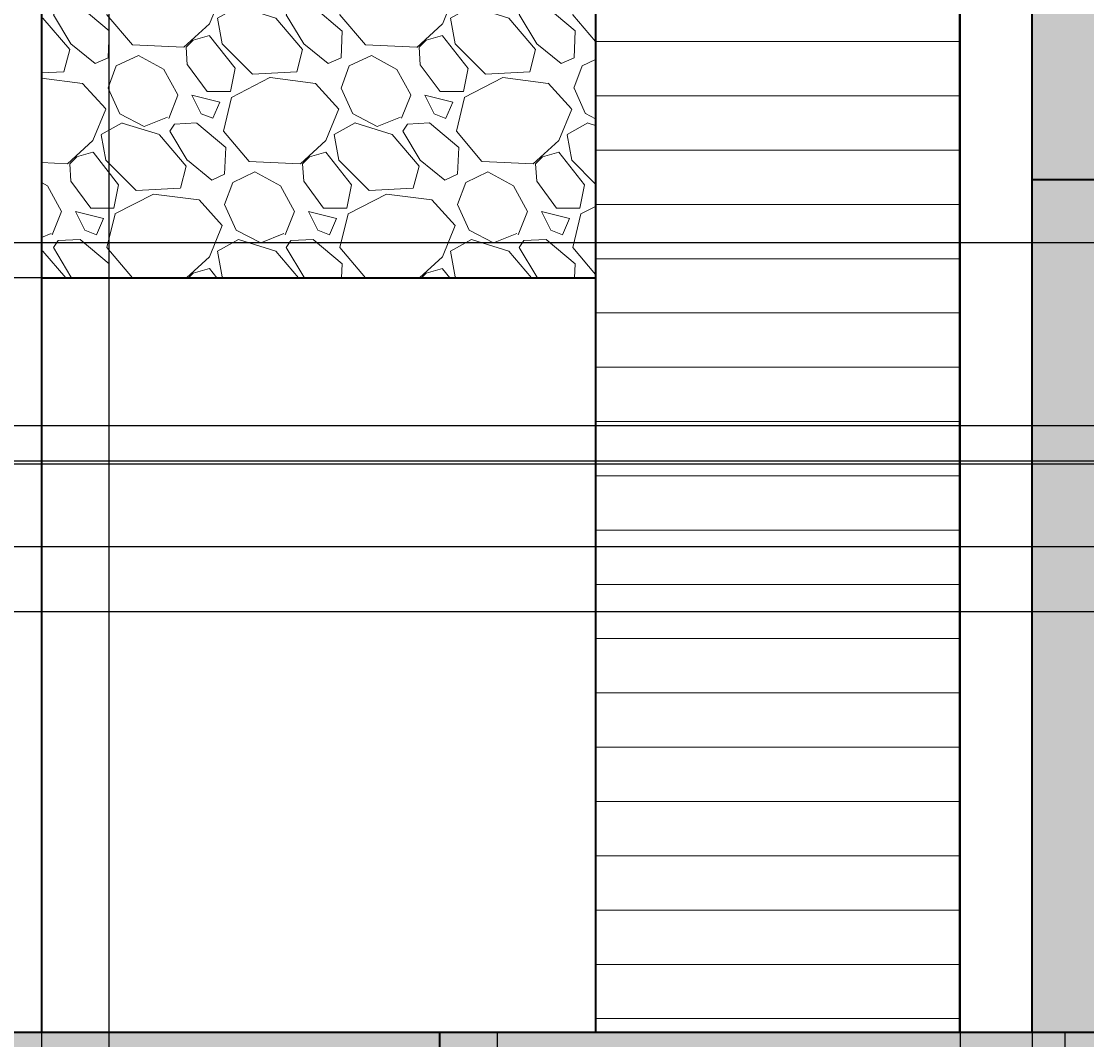
# Model space of a CAD drawing. Units: inches. Extents: x -5 to 714, y 84 to 644.
# Tile 4 of 20: x 124 to 266, y 200 to 336. Entities that reach past the tile are written whole.
import ezdxf

# ---------------------------------------------------------------- set-up
doc = ezdxf.new("R2010")
doc.units = ezdxf.units.IN
doc.header["$MEASUREMENT"] = 0
for name, color, linetype, lineweight in [('A-ANNO-DIMS', 2, 'Continuous', 18), ('A-ELEV', 7, 'Continuous', 35), ('A-ELEV-PATT', 8, 'Continuous', 13), ('A-GLAZ', 3, 'Continuous', 25)]:
    doc.layers.add(name, color=color, linetype=linetype, lineweight=lineweight)
doc.styles.get("Standard").update_dxf_attribs({"font": 'arial.ttf'})
doc.dimstyles.get("Standard").update_dxf_attribs({"dimtxt": 0.9375, "dimasz": 0.18, "dimexe": 0.18, "dimexo": 0.0625, "dimgap": 0.09, "dimtad": 0, "dimtih": 1, "dimtoh": 1, "dimdec": 4, "dimzin": 0, "dimdsep": 46, "dimlunit": 4, "dimtxsty": 'Standard', "dimcen": 0.09, "dimadec": 0, "dimazin": 0, "dimtfac": 1, "dimtdec": 4, "dimtofl": 0, "dimtmove": 0, "dimatfit": 3, "dimfxl": 1, "dimtolj": 1, "dimtzin": 0, "dimarcsym": 0})

# ---------------------------------------------------------------- blocks, each defined once
blk = doc.blocks.new('*D28')
at = {"layer": 'A-ANNO-DIMS', "color": 0, "lineweight": -2, "transparency": 16777216}
for p, q in [((126.73, 480.11), (126.73, 84.31)), ((135.73, 471.11), (135.73, 84.31)), ((126.91, 84.49), (130.83, 84.49)), ((135.55, 84.49), (131.63, 84.49))]:
    blk.add_line(p, q, dxfattribs=at)
at = {"layer": 'A-ANNO-DIMS', "color": 0, "transparency": 16777216}
for points in [[(126.91, 84.52), (126.91, 84.46), (126.73, 84.49)], [(135.55, 84.52), (135.55, 84.46), (135.73, 84.49)]]:
    blk.add_solid(points, dxfattribs=at)
at = {"layer": 'Defpoints', "color": 0, "transparency": 16777216}
for p in [(126.73, 480.17), (135.73, 471.17), (135.73, 84.49)]:
    blk.add_point(p, dxfattribs=at)
at = {"layer": 'A-ANNO-DIMS', "color": 0, "transparency": 16777216, "insert": (131.23, 84.49), "char_height": 0.938, "attachment_point": 5}
blk.add_mtext('\\A1;9', dxfattribs=at)
blk = doc.blocks.new('*D29')
at = {"layer": 'A-ANNO-DIMS', "color": 0, "lineweight": -2, "transparency": 16777216}
for p, q in [((135.73, 471.11), (135.73, 84.31)), ((429.51, 471.11), (429.51, 84.31)), ((135.91, 84.49), (280.94, 84.49)), ((429.33, 84.49), (284.3, 84.49))]:
    blk.add_line(p, q, dxfattribs=at)
at = {"layer": 'A-ANNO-DIMS', "color": 0, "transparency": 16777216}
for points in [[(135.91, 84.52), (135.91, 84.46), (135.73, 84.49)], [(429.33, 84.52), (429.33, 84.46), (429.51, 84.49)]]:
    blk.add_solid(points, dxfattribs=at)
at = {"layer": 'Defpoints', "color": 0, "transparency": 16777216}
for p in [(135.73, 471.17), (429.51, 471.17), (429.51, 84.49)]:
    blk.add_point(p, dxfattribs=at)
at = {"layer": 'A-ANNO-DIMS', "color": 0, "transparency": 16777216, "insert": (282.62, 84.49), "char_height": 0.938, "attachment_point": 5}
blk.add_mtext('\\A1;293.8', dxfattribs=at)
blk = doc.blocks.new('*D49')
at = {"layer": 'A-ANNO-DIMS', "color": 0, "lineweight": -2, "transparency": 16777216}
for p, q in [((126.73, 302), (126.73, 643.61)), ((126.91, 643.43), (162.98, 643.43)), ((200.56, 643.43), (164.49, 643.43)), ((200.74, 302), (200.74, 643.61))]:
    blk.add_line(p, q, dxfattribs=at)
at = {"layer": 'A-ANNO-DIMS', "color": 0, "transparency": 16777216}
for points in [[(126.91, 643.46), (126.91, 643.4), (126.73, 643.43)], [(200.56, 643.46), (200.56, 643.4), (200.74, 643.43)]]:
    blk.add_solid(points, dxfattribs=at)
at = {"layer": 'Defpoints', "color": 0, "transparency": 16777216}
for p in [(200.74, 643.43), (126.73, 301.94), (200.74, 301.94)]:
    blk.add_point(p, dxfattribs=at)
at = {"layer": 'A-ANNO-DIMS', "color": 0, "transparency": 16777216, "insert": (163.73, 643.43), "char_height": 0.938, "attachment_point": 5}
blk.add_mtext('\\A1;74', dxfattribs=at)
blk = doc.blocks.new('*D50')
at = {"layer": 'A-ANNO-DIMS', "color": 0, "lineweight": -2, "transparency": 16777216}
for p, q in [((200.67, 345.19), (-2.74, 345.19)), ((-2.56, 345.01), (-2.56, 324.13)), ((-2.56, 302.12), (-2.56, 323)), ((200.67, 301.94), (-2.74, 301.94))]:
    blk.add_line(p, q, dxfattribs=at)
at = {"layer": 'A-ANNO-DIMS', "color": 0, "transparency": 16777216}
for points in [[(-2.59, 345.01), (-2.53, 345.01), (-2.56, 345.19)], [(-2.59, 302.12), (-2.53, 302.12), (-2.56, 301.94)]]:
    blk.add_solid(points, dxfattribs=at)
at = {"layer": 'Defpoints', "color": 0, "transparency": 16777216}
for p in [(-2.56, 345.19), (200.74, 345.19), (200.74, 301.94)]:
    blk.add_point(p, dxfattribs=at)
at = {"layer": 'A-ANNO-DIMS', "color": 0, "transparency": 16777216, "insert": (-2.56, 323.57), "char_height": 0.938, "attachment_point": 5}
blk.add_mtext('\\A1;43.255', dxfattribs=at)
blk = doc.blocks.new('*D51')
at = {"layer": 'A-ANNO-DIMS', "color": 0, "lineweight": -2, "transparency": 16777216}
for p, q in [((200.74, 201.26), (200.74, 643.61)), ((200.92, 643.43), (223.39, 643.43)), ((249.24, 643.43), (226.77, 643.43)), ((249.42, 201.26), (249.42, 643.61))]:
    blk.add_line(p, q, dxfattribs=at)
at = {"layer": 'A-ANNO-DIMS', "color": 0, "transparency": 16777216}
for points in [[(200.92, 643.46), (200.92, 643.4), (200.74, 643.43)], [(249.24, 643.46), (249.24, 643.4), (249.42, 643.43)]]:
    blk.add_solid(points, dxfattribs=at)
at = {"layer": 'Defpoints', "color": 0, "transparency": 16777216}
for p in [(249.42, 643.43), (200.74, 201.19), (249.42, 201.19)]:
    blk.add_point(p, dxfattribs=at)
at = {"layer": 'A-ANNO-DIMS', "color": 0, "transparency": 16777216, "insert": (225.08, 643.43), "char_height": 0.938, "attachment_point": 5}
blk.add_mtext('\\A1;48.68', dxfattribs=at)
blk = doc.blocks.new('*D52')
at = {"layer": 'A-ANNO-DIMS', "color": 0, "lineweight": -2, "transparency": 16777216}
for p, q in [((249.42, 345.13), (249.42, 84.31)), ((259.07, 345.13), (259.07, 84.31)), ((249.6, 84.49), (252.57, 84.49)), ((258.89, 84.49), (255.92, 84.49))]:
    blk.add_line(p, q, dxfattribs=at)
at = {"layer": 'A-ANNO-DIMS', "color": 0, "transparency": 16777216}
for points in [[(249.6, 84.52), (249.6, 84.46), (249.42, 84.49)], [(258.89, 84.52), (258.89, 84.46), (259.07, 84.49)]]:
    blk.add_solid(points, dxfattribs=at)
at = {"layer": 'Defpoints', "color": 0, "transparency": 16777216}
for p in [(249.42, 345.19), (259.07, 345.19), (259.07, 84.49)]:
    blk.add_point(p, dxfattribs=at)
at = {"layer": 'A-ANNO-DIMS', "color": 0, "transparency": 16777216, "insert": (254.24, 84.49), "char_height": 0.938, "attachment_point": 5}
blk.add_mtext('\\A1;9.648', dxfattribs=at)
blk = doc.blocks.new('*D53')
at = {"layer": 'A-ANNO-DIMS', "color": 0, "lineweight": -2, "transparency": 16777216}
for p, q in [((259.07, 315.03), (259.07, 84.31)), ((269.24, 306.57), (269.24, 84.31)), ((259.25, 84.49), (262.16, 84.49)), ((269.06, 84.49), (266.15, 84.49))]:
    blk.add_line(p, q, dxfattribs=at)
at = {"layer": 'A-ANNO-DIMS', "color": 0, "transparency": 16777216}
for points in [[(259.25, 84.52), (259.25, 84.46), (259.07, 84.49)], [(269.06, 84.52), (269.06, 84.46), (269.24, 84.49)]]:
    blk.add_solid(points, dxfattribs=at)
at = {"layer": 'Defpoints', "color": 0, "transparency": 16777216}
for p in [(259.07, 315.1), (269.24, 306.63), (269.24, 84.49)]:
    blk.add_point(p, dxfattribs=at)
at = {"layer": 'A-ANNO-DIMS', "color": 0, "transparency": 16777216, "insert": (264.16, 84.49), "char_height": 0.938, "attachment_point": 5}
blk.add_mtext('\\A1;10.178', dxfattribs=at)
blk = doc.blocks.new('*D54')
at = {"layer": 'A-ANNO-DIMS', "color": 0, "lineweight": -2, "transparency": 16777216}
for p, q in [((259.07, 315.16), (259.07, 643.61)), ((259.25, 643.43), (424.21, 643.43)), ((593.25, 643.43), (428.28, 643.43)), ((593.43, 315.16), (593.43, 643.61))]:
    blk.add_line(p, q, dxfattribs=at)
at = {"layer": 'A-ANNO-DIMS', "color": 0, "transparency": 16777216}
for points in [[(259.25, 643.46), (259.25, 643.4), (259.07, 643.43)], [(593.25, 643.46), (593.25, 643.4), (593.43, 643.43)]]:
    blk.add_solid(points, dxfattribs=at)
at = {"layer": 'Defpoints', "color": 0, "transparency": 16777216}
for p in [(593.43, 643.43), (259.07, 315.1), (593.43, 315.1)]:
    blk.add_point(p, dxfattribs=at)
at = {"layer": 'A-ANNO-DIMS', "color": 0, "transparency": 16777216, "insert": (426.25, 643.43), "char_height": 0.938, "attachment_point": 5}
blk.add_mtext('\\A1;334.36', dxfattribs=at)
blk = doc.blocks.new('*D56')
at = {"layer": 'A-ANNO-DIMS', "color": 0, "lineweight": -2, "transparency": 16777216}
for p, q in [((578.03, 277.05), (-2.74, 277.05)), ((-2.56, 276.87), (-2.56, 239.69)), ((-2.56, 201.37), (-2.56, 238.55)), ((578.03, 201.19), (-2.74, 201.19))]:
    blk.add_line(p, q, dxfattribs=at)
at = {"layer": 'A-ANNO-DIMS', "color": 0, "transparency": 16777216}
for points in [[(-2.59, 276.87), (-2.53, 276.87), (-2.56, 277.05)], [(-2.59, 201.37), (-2.53, 201.37), (-2.56, 201.19)]]:
    blk.add_solid(points, dxfattribs=at)
at = {"layer": 'Defpoints', "color": 0, "transparency": 16777216}
for p in [(-2.56, 277.05), (578.09, 277.05), (578.09, 201.19)]:
    blk.add_point(p, dxfattribs=at)
at = {"layer": 'A-ANNO-DIMS', "color": 0, "transparency": 16777216, "insert": (-2.56, 239.12), "char_height": 0.938, "attachment_point": 5}
blk.add_mtext('\\A1;75.86', dxfattribs=at)
blk = doc.blocks.new('*D57')
at = {"layer": 'A-ANNO-DIMS', "color": 0, "lineweight": -2, "transparency": 16777216}
for p, q in [((578.03, 306.63), (-2.74, 306.63)), ((-2.56, 306.45), (-2.56, 292.41)), ((-2.56, 277.23), (-2.56, 291.27)), ((578.03, 277.05), (-2.74, 277.05))]:
    blk.add_line(p, q, dxfattribs=at)
at = {"layer": 'A-ANNO-DIMS', "color": 0, "transparency": 16777216}
for points in [[(-2.59, 306.45), (-2.53, 306.45), (-2.56, 306.63)], [(-2.59, 277.23), (-2.53, 277.23), (-2.56, 277.05)]]:
    blk.add_solid(points, dxfattribs=at)
at = {"layer": 'Defpoints', "color": 0, "transparency": 16777216}
for p in [(578.09, 306.63), (-2.56, 277.05), (578.09, 277.05)]:
    blk.add_point(p, dxfattribs=at)
at = {"layer": 'A-ANNO-DIMS', "color": 0, "transparency": 16777216, "insert": (-2.56, 291.84), "char_height": 0.938, "attachment_point": 5}
blk.add_mtext('\\A1;29.58', dxfattribs=at)
blk = doc.blocks.new('*D59')
at = {"layer": 'A-ANNO-DIMS', "color": 0, "lineweight": -2, "transparency": 16777216}
for p, q in [((593.37, 282.2), (-2.74, 282.2)), ((-2.56, 282.02), (-2.56, 280.41)), ((-2.56, 277.66), (-2.56, 279.27)), ((593.37, 277.48), (-2.74, 277.48))]:
    blk.add_line(p, q, dxfattribs=at)
at = {"layer": 'A-ANNO-DIMS', "color": 0, "transparency": 16777216}
for points in [[(-2.59, 282.02), (-2.53, 282.02), (-2.56, 282.2)], [(-2.59, 277.66), (-2.53, 277.66), (-2.56, 277.48)]]:
    blk.add_solid(points, dxfattribs=at)
at = {"layer": 'Defpoints', "color": 0, "transparency": 16777216}
for p in [(-2.56, 282.2), (593.43, 282.2), (593.43, 277.48)]:
    blk.add_point(p, dxfattribs=at)
at = {"layer": 'A-ANNO-DIMS', "color": 0, "transparency": 16777216, "insert": (-2.56, 279.84), "char_height": 0.938, "attachment_point": 5}
blk.add_mtext('\\A1;4.719', dxfattribs=at)
blk = doc.blocks.new('*D65')
at = {"layer": 'A-ANNO-DIMS', "color": 0, "lineweight": -2, "transparency": 16777216}
for p, q in [((325.77, 266), (-2.74, 266)), ((-2.56, 265.82), (-2.56, 219.13)), ((-2.56, 171.3), (-2.56, 217.99)), ((325.77, 171.12), (-2.74, 171.12))]:
    blk.add_line(p, q, dxfattribs=at)
at = {"layer": 'A-ANNO-DIMS', "color": 0, "transparency": 16777216}
for points in [[(-2.59, 265.82), (-2.53, 265.82), (-2.56, 266)], [(-2.59, 171.3), (-2.53, 171.3), (-2.56, 171.12)]]:
    blk.add_solid(points, dxfattribs=at)
at = {"layer": 'Defpoints', "color": 0, "transparency": 16777216}
for p in [(-2.56, 266), (325.83, 266), (325.83, 171.12)]:
    blk.add_point(p, dxfattribs=at)
at = {"layer": 'A-ANNO-DIMS', "color": 0, "transparency": 16777216, "insert": (-2.56, 218.56), "char_height": 0.938, "attachment_point": 5}
blk.add_mtext('\\A1;94.88', dxfattribs=at)
blk = doc.blocks.new('*D71')
at = {"layer": 'A-ANNO-DIMS', "color": 0, "lineweight": -2, "transparency": 16777216}
for p, q in [((537.12, 257.34), (-2.74, 257.34)), ((-2.56, 257.16), (-2.56, 229.83)), ((-2.56, 201.37), (-2.56, 228.7)), ((537.12, 201.19), (-2.74, 201.19))]:
    blk.add_line(p, q, dxfattribs=at)
at = {"layer": 'A-ANNO-DIMS', "color": 0, "transparency": 16777216}
for points in [[(-2.59, 257.16), (-2.53, 257.16), (-2.56, 257.34)], [(-2.59, 201.37), (-2.53, 201.37), (-2.56, 201.19)]]:
    blk.add_solid(points, dxfattribs=at)
at = {"layer": 'Defpoints', "color": 0, "transparency": 16777216}
for p in [(-2.56, 257.34), (537.18, 257.34), (537.18, 201.19)]:
    blk.add_point(p, dxfattribs=at)
at = {"layer": 'A-ANNO-DIMS', "color": 0, "transparency": 16777216, "insert": (-2.56, 229.27), "char_height": 0.938, "attachment_point": 5}
blk.add_mtext('\\A1;56.15', dxfattribs=at)
blk = doc.blocks.new('*D72')
at = {"layer": 'A-ANNO-DIMS', "color": 0, "lineweight": -2, "transparency": 16777216}
for p, q in [((493.71, 266), (-2.74, 266)), ((-2.56, 265.82), (-2.56, 234.17)), ((-2.56, 201.37), (-2.56, 233.03)), ((493.71, 201.19), (-2.74, 201.19))]:
    blk.add_line(p, q, dxfattribs=at)
at = {"layer": 'A-ANNO-DIMS', "color": 0, "transparency": 16777216}
for points in [[(-2.59, 265.82), (-2.53, 265.82), (-2.56, 266)], [(-2.59, 201.37), (-2.53, 201.37), (-2.56, 201.19)]]:
    blk.add_solid(points, dxfattribs=at)
at = {"layer": 'Defpoints', "color": 0, "transparency": 16777216}
for p in [(-2.56, 266), (493.78, 266), (493.78, 201.19)]:
    blk.add_point(p, dxfattribs=at)
at = {"layer": 'A-ANNO-DIMS', "color": 0, "transparency": 16777216, "insert": (-2.56, 233.6), "char_height": 0.938, "attachment_point": 5}
blk.add_mtext('\\A1;64.81', dxfattribs=at)
blk = doc.blocks.new('*D82')
at = {"layer": 'A-ANNO-DIMS', "color": 0, "lineweight": -2, "transparency": 16777216}
for p, q in [((263.37, 201.19), (-2.74, 201.19)), ((-2.56, 201.01), (-2.56, 177.22)), ((-2.56, 152.3), (-2.56, 176.09)), ((263.37, 152.12), (-2.74, 152.12))]:
    blk.add_line(p, q, dxfattribs=at)
at = {"layer": 'A-ANNO-DIMS', "color": 0, "transparency": 16777216}
for points in [[(-2.59, 201.01), (-2.53, 201.01), (-2.56, 201.19)], [(-2.59, 152.3), (-2.53, 152.3), (-2.56, 152.12)]]:
    blk.add_solid(points, dxfattribs=at)
at = {"layer": 'Defpoints', "color": 0, "transparency": 16777216}
for p in [(-2.56, 201.19), (263.43, 201.19), (263.43, 152.12)]:
    blk.add_point(p, dxfattribs=at)
at = {"layer": 'A-ANNO-DIMS', "color": 0, "transparency": 16777216, "insert": (-2.56, 176.66), "char_height": 0.938, "attachment_point": 5}
blk.add_mtext('\\A1;49.08', dxfattribs=at)

msp = doc.modelspace()

# ---------------------------------------------------------------- hatches: boundary and pattern name
at = {"layer": 'A-ELEV-PATT', "transparency": 33554687}
h = msp.add_hatch(color=256, dxfattribs=at)
h.dxf.hatch_style = 1
h.paths.add_polyline_path([(188.3677, 525.1928), (67.9893, 525.1928), (67.9893, 489.1928), (67.9893, 345.1928), (126.7303, 345.1928), (126.7303, 480.1709), (229.3575, 480.1709), (229.3575, 525.1928), (212.6043, 525.1928), (212.6043, 482.7164), (211.0019, 482.7164), (211.0019, 525.1928), (207.6919, 525.1928), (199.9852, 525.1928), (199.9852, 482.7164), (198.3828, 482.7164), (198.3828, 525.1928), (189.9701, 525.1928), (189.9701, 482.7164), (188.3677, 482.7164)])
h.paths.add_polyline_path([(121.3589, 336.2066), (75.5048, 336.2066), (75.5048, 319.345), (121.3589, 319.345)])
h.paths.add_polyline_path([(121.3589, 319.345), (75.5048, 319.345), (75.5048, 302.3045), (121.3589, 302.3045)])
h.paths.add_polyline_path([(121.3589, 302.3045), (75.5048, 302.3045), (75.5048, 282.8561), (121.3589, 282.8561)])
h.paths.add_polyline_path([(121.3589, 282.8561), (75.5048, 282.8561), (75.5048, 261.5556), (121.3589, 261.5556)])
h.paths.add_polyline_path([(121.3589, 261.5556), (75.5048, 261.5556), (75.5048, 243.7009), (121.3589, 243.7009)])
h.paths.add_polyline_path([(121.3589, 243.7009), (75.5048, 243.7009), (75.5048, 223.5117), (121.3589, 223.5117)])
h.paths.add_polyline_path([(121.3589, 223.5117), (75.5048, 223.5117), (75.5048, 212.5836), (121.3589, 212.5836)])
h.paths.add_polyline_path([(121.3589, 212.5836), (75.5048, 212.5836), (75.5048, 201.1928), (121.3589, 201.1928)])
h.paths.add_polyline_path([(179.9335, 201.1928), (30.1395, 201.1928), (30.1395, 198.7054), (179.9335, 198.7054)])
h.paths.add_polyline_path([(187.6349, 201.1928), (179.9335, 201.1928), (179.9335, 198.7054), (179.9335, 141.1928), (269.2446, 141.1928), (269.2446, 201.1928), (263.4349, 201.1928), (263.4349, 152.1176), (187.6349, 152.1176)])
h.paths.add_polyline_path([(269.2446, 277.0513), (269.2446, 287.501), (269.2446, 306.6286), (578.0915, 306.6286), (578.0915, 201.1928), (593.428, 201.1928), (593.428, 315.0968), (584.4202, 315.0968), (259.0665, 315.0968), (259.0665, 201.1928), (263.4349, 201.1928), (269.2446, 201.1928)])
h = msp.add_hatch(dxfattribs=at)
h.set_pattern_fill('ANSI31', color=256, scale=58, angle=135)
h.paths.add_polyline_path([(249.4181, 345.1928), (237.2654, 345.1928), (200.7361, 345.1928), (200.7361, 201.1928), (249.4181, 201.1928)])
h.paths.add_polyline_path([(261.4349, 199.1928), (189.6349, 199.1928), (189.6349, 154.1176), (261.4349, 154.1176)])
h.paths.add_polyline_path([(415.8092, 525.1928), (366.2809, 525.1928), (366.2809, 480.1709), (415.8092, 480.1709)])
h = msp.add_hatch(dxfattribs=at)
h.set_pattern_fill('GRAVEL', color=256, scale=22, angle=135)
h.paths.add_polyline_path([(200.7361, 345.1928), (126.7303, 345.1928), (126.7303, 301.9374), (200.7361, 301.9374)])
h = msp.add_hatch(color=256, dxfattribs=at)
h.dxf.hatch_style = 1
h.paths.add_polyline_path([(584.2229, 343.1928), (259.0665, 343.1928), (259.0665, 315.0968), (584.2229, 315.0968)])
h.paths.add_polyline_path([(352.9482, 258.2864), (332.0052, 258.2864), (332.0052, 201.1928), (352.9482, 201.1928)])
h.paths.add_polyline_path([(378.5957, 258.2864), (357.6527, 258.2864), (357.6527, 201.1928), (378.5957, 201.1928)])
h.paths.add_polyline_path([(403.4391, 258.2864), (382.4961, 258.2864), (382.4961, 201.1928), (403.4391, 201.1928)])
h.paths.add_polyline_path([(339.2672, 197.3754), (332.0052, 197.3754), (332.0052, 191.3028), (339.2672, 191.3028)])
h.paths.add_polyline_path([(352.9482, 197.3754), (343.9704, 197.3754), (343.9704, 191.3028), (352.9482, 191.3028)])
h.paths.add_polyline_path([(352.9482, 189.3028), (343.9704, 189.3028), (343.9704, 184.8307), (352.9482, 184.8307)])
h.paths.add_polyline_path([(339.2672, 189.3028), (332.0052, 189.3028), (332.0052, 184.8307), (339.2672, 184.8307)])
h.paths.add_polyline_path([(339.2672, 182.8307), (332.0052, 182.8307), (332.0052, 177.6504), (339.2672, 177.6504)])
h.paths.add_polyline_path([(352.9482, 182.8307), (343.9704, 182.8307), (343.9704, 177.6504), (352.9482, 177.6504)])
h.paths.add_polyline_path([(352.9482, 175.6504), (343.9704, 175.6504), (343.9704, 173.6169), (352.9482, 173.6169)])
h.paths.add_polyline_path([(339.2672, 175.6504), (332.0052, 175.6504), (332.0052, 173.6169), (339.2672, 173.6169)])
h.paths.add_polyline_path([(376.2796, 175.6504), (357.6527, 175.6504), (357.6527, 173.6169), (376.2796, 173.6169)])
h.paths.add_polyline_path([(376.2796, 182.8307), (357.6527, 182.8307), (357.6527, 177.6504), (376.2796, 177.6504)])
h.paths.add_polyline_path([(376.2796, 189.3028), (357.6527, 189.3028), (357.6527, 184.8307), (376.2796, 184.8307)])
h.paths.add_polyline_path([(376.2796, 197.3754), (357.6527, 197.3754), (357.6527, 191.3028), (376.2796, 191.3028)])
h.paths.add_polyline_path([(403.4391, 197.3754), (382.4961, 197.3754), (382.4961, 191.3028), (403.4391, 191.3028)])
h.paths.add_polyline_path([(403.4391, 189.3028), (382.4961, 189.3028), (382.4961, 184.8307), (403.4391, 184.8307)])
h.paths.add_polyline_path([(403.4391, 182.8307), (382.4961, 182.8307), (382.4961, 177.6504), (403.4391, 177.6504)])
h.paths.add_polyline_path([(403.4391, 175.6504), (382.4961, 175.6504), (382.4961, 173.6169), (403.4391, 173.6169)])
h = msp.add_hatch(color=256, dxfattribs=at)
h.dxf.hatch_style = 1
h.paths.add_polyline_path([(263.4349, 201.1928), (187.6349, 201.1928), (187.6349, 152.1176), (263.4349, 152.1176)])
h.paths.add_polyline_path([(189.6349, 199.1928), (261.4349, 199.1928), (261.4349, 154.1176), (189.6349, 154.1176)], flags=16)

# ---------------------------------------------------------------- linework, layer by layer
at = {"layer": 'A-ELEV'}
for p, q in [((126.7303, 345.1928), (126.7303, 201.1928)), ((200.7361, 345.1928), (200.7361, 201.1928)), ((249.4181, 201.1928), (249.4181, 345.1928)), ((259.0665, 201.1928), (259.0665, 345.1928)), ((259.0665, 315.0968), (584.4202, 315.0968)), ((126.7303, 301.9374), (200.7361, 301.9374)), ((30.1395, 201.1928), (545.1065, 201.1928)), ((179.9335, 198.7054), (179.9335, 201.1928))]:
    msp.add_line(p, q, dxfattribs=at)
at = {"layer": 'A-GLAZ'}
msp.add_lwpolyline([(187.6349, 201.1928), (263.4349, 201.1928), (263.4349, 152.1176), (187.6349, 152.1176)], close=True, dxfattribs=at)

# ---------------------------------------------------------------- dimensions: what is measured, and where the dimension line sits
at = {"layer": 'A-ANNO-DIMS'}
for base, p1, p2, override, picture, middle in [((200.7361, 643.4276), (126.7303, 301.9374), (200.7361, 301.9374), {"dimdec": 0, "dimlfac": 1, "dimrnd": 0, "dimzin": 0, "dimdsep": 46, "dimlunit": 2}, '*D49', (163.7332, 643.4276)), ((249.4181, 643.4276), (200.7361, 201.1928), (249.4181, 201.1928), {"dimdec": 2, "dimlfac": 1, "dimrnd": 0, "dimzin": 0, "dimdsep": 46, "dimlunit": 2}, '*D51', (225.0771, 643.4276)), ((593.428, 643.4276), (259.0665, 315.0968), (593.428, 315.0968), {"dimdec": 2, "dimlfac": 1, "dimrnd": 0, "dimzin": 0, "dimdsep": 46, "dimlunit": 2}, '*D54', (426.2472, 643.4276)), ((135.7303, 84.4928), (126.7303, 480.1709), (135.7303, 471.1709), {"dimdec": 0, "dimlfac": 1, "dimrnd": 0, "dimzin": 0, "dimdsep": 46, "dimlunit": 2}, '*D28', (131.2303, 84.4928)), ((429.5094, 84.4928), (135.7303, 471.1709), (429.5094, 471.1709), {"dimdec": 1, "dimlfac": 1, "dimrnd": 0, "dimzin": 0, "dimdsep": 46, "dimlunit": 2}, '*D29', (282.6198, 84.4928)), ((259.0665, 84.4928), (249.4181, 345.1928), (259.0665, 345.1928), {"dimdec": 3, "dimlfac": 1, "dimrnd": 0, "dimzin": 0, "dimdsep": 46, "dimlunit": 2}, '*D52', (254.2423, 84.4928)), ((269.2446, 84.4928), (259.0665, 315.0968), (269.2446, 306.6286), {"dimdec": 3, "dimlfac": 1, "dimrnd": 0, "dimzin": 0, "dimdsep": 46, "dimlunit": 2}, '*D53', (264.1555, 84.4928))]:
    dim = msp.add_linear_dim(base=base, p1=p1, p2=p2, dimstyle='Standard', override=override, dxfattribs=at)
    dim.commit()
    dim.dimension.update_dxf_attribs({"geometry": picture, "text_midpoint": middle})
for base, p1, p2, override, picture, middle in [((-2.5605, 345.1928), (200.7361, 301.9374), (200.7361, 345.1928), {"dimdec": 3, "dimlfac": 1, "dimrnd": 0, "dimzin": 0, "dimdsep": 46, "dimlunit": 2}, '*D50', (-2.5605, 323.5651)), ((-2.5605, 277.0513), (578.0915, 306.6286), (578.0915, 277.0513), {"dimdec": 2, "dimlfac": 1, "dimrnd": 0, "dimzin": 0, "dimdsep": 46, "dimlunit": 2}, '*D57', (-2.5605, 291.84)), ((-2.5605, 282.1969), (593.428, 277.4776), (593.428, 282.1969), {"dimdec": 3, "dimlfac": 1, "dimrnd": 0, "dimzin": 0, "dimdsep": 46, "dimlunit": 2}, '*D59', (-2.5605, 279.8372)), ((-2.5605, 277.0513), (578.0915, 201.1928), (578.0915, 277.0513), {"dimdec": 2, "dimlfac": 1, "dimrnd": 0, "dimzin": 0, "dimdsep": 46, "dimlunit": 2}, '*D56', (-2.5605, 239.1221)), ((-2.5605, 266.0021), (325.8305, 171.1197), (325.8305, 266.0021), {"dimdec": 2, "dimlfac": 1, "dimrnd": 0, "dimzin": 0, "dimdsep": 46, "dimlunit": 2}, '*D65', (-2.5605, 218.5609)), ((-2.5605, 266.0021), (493.7771, 201.1928), (493.7771, 266.0021), {"dimdec": 2, "dimlfac": 1, "dimrnd": 0, "dimzin": 0, "dimdsep": 46, "dimlunit": 2}, '*D72', (-2.5605, 233.5974)), ((-2.5605, 257.3379), (537.1779, 201.1928), (537.1779, 257.3379), {"dimdec": 2, "dimlfac": 1, "dimrnd": 0, "dimzin": 0, "dimdsep": 46, "dimlunit": 2}, '*D71', (-2.5605, 229.2653)), ((-2.5605, 201.1928), (263.4349, 152.1176), (263.4349, 201.1928), {"dimdec": 2, "dimlfac": 1, "dimrnd": 0, "dimzin": 0, "dimdsep": 46, "dimlunit": 2}, '*D82', (-2.5605, 176.6552))]:
    dim = msp.add_linear_dim(base=base, p1=p1, p2=p2, angle=90, dimstyle='Standard', override=override, dxfattribs=at)
    dim.commit()
    dim.dimension.update_dxf_attribs({"geometry": picture, "text_midpoint": middle})

doc.saveas('drawing.dxf')
